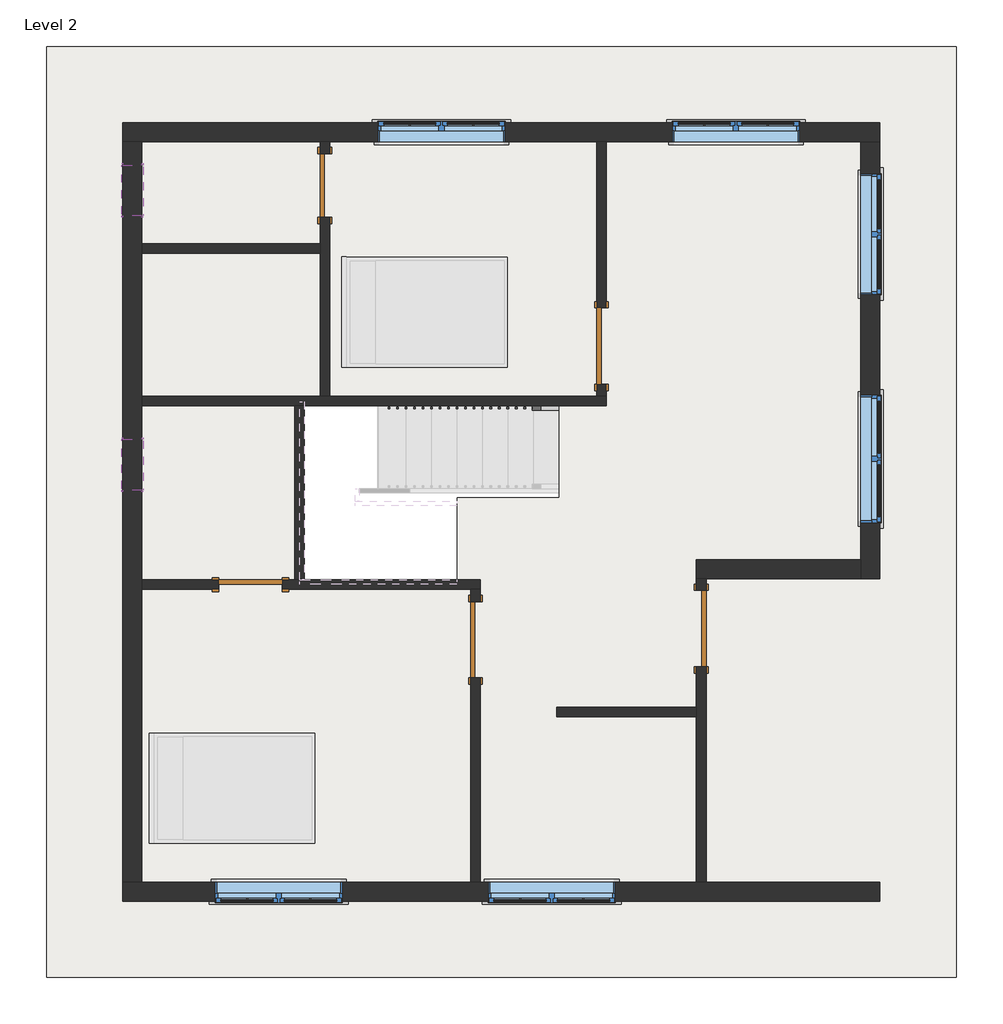
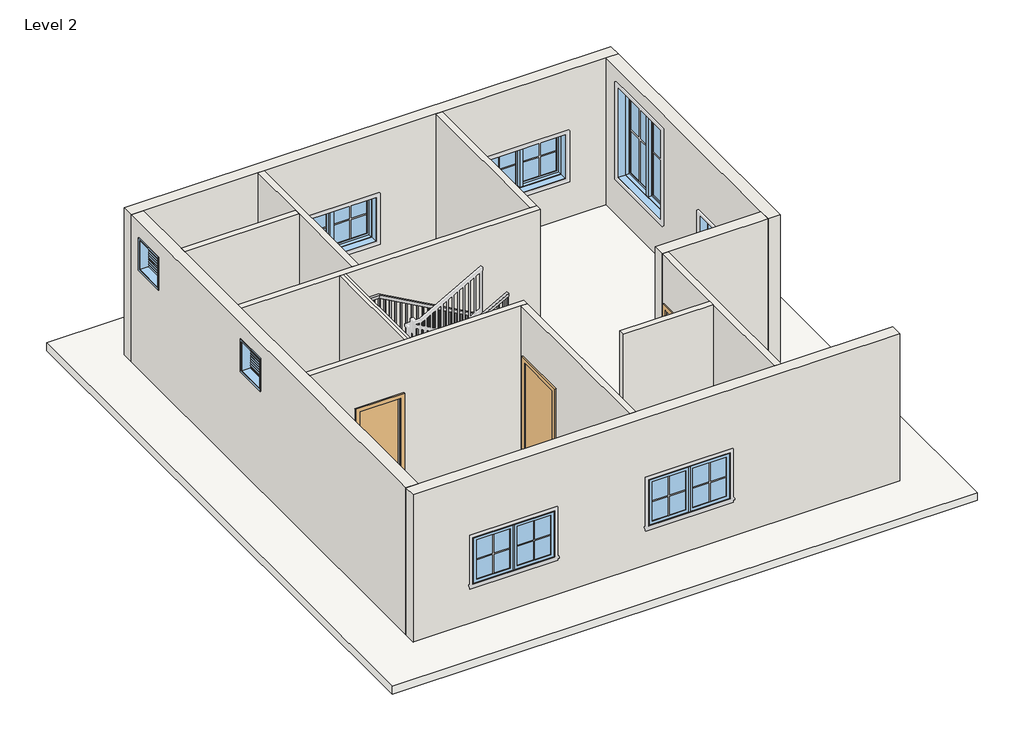
# One storey, part 1 of 2: 14 walls, 8 windows, 5 doors, 1 railing, 1 roof.
"""IFC4 building model written with IfcOpenShell, lengths in millimetres."""

from ifc_helpers import new_model, si_unit, frame, origin, place, context, project, spatial, polyline, outline, extrude, faceted_brep, transform, mapped, element, save
from components import single_flush_3_17d80c48, single_flush_3_5e62189b, door_d8f5dbb5, window_9ac97e1a, window_c1d95f0f, window_f2d8fef0

model = new_model("IFC4")

# Units and contexts
model_context = context("Model", 3, world=origin())
ifc_project = project(units=[si_unit("LENGTHUNIT", "METRE", prefix="MILLI")], contexts=[model_context])

# Site, building, storey
site = spatial("IfcSite", under=ifc_project)
building = spatial("IfcBuilding", under=site)
storey = spatial("IfcBuildingStorey", under=building, Name="Level 2", Elevation=3048.0)

# Doors
placement = place(None, origin())
single_flush_3_shape = single_flush_3_17d80c48(model_context)
element("IfcDoor", 1, ObjectType="Single-Flush : 3'", at=placement, inside=storey, context=model_context, shape_type="MappedRepresentation", body=[
    mapped(single_flush_3_shape, transform((-1566.5130704, -2143.0042021, 3048.0), x_axis=(0.0, 1.0, 0.0), y_axis=(-1.0, 0.0, 0.0), z_axis=(0.0, 0.0, 1.0))),
])
single_flush_3_2_shape = single_flush_3_5e62189b(model_context)
element("IfcDoor", 2, ObjectType="Single-Flush : 3'", at=placement, inside=storey, context=model_context, shape_type="MappedRepresentation", body=[
    mapped(single_flush_3_2_shape, transform((1138.5869296, -2009.6542021, 3048.0), x_axis=(0.0, 1.0, 0.0), y_axis=(-1.0, 0.0, 0.0), z_axis=(0.0, 0.0, 1.0))),
])
element("IfcDoor", 3, ObjectType="Single-Flush : 3'", at=placement, inside=storey, context=model_context, shape_type="MappedRepresentation", body=[
    mapped(single_flush_3_2_shape, transform((-55.2130704, 1374.8957979, 3048.0), x_axis=(0.0, -1.0, 0.0), y_axis=(1.0, 0.0, 0.0), z_axis=(0.0, 0.0, 1.0))),
])
door_shape = door_d8f5dbb5(model_context)
element("IfcDoor", 4, ObjectType="Single-Flush : DOOR 2'6\"", at=placement, inside=storey, context=model_context, shape_type="MappedRepresentation", body=[
    mapped(door_shape, transform((-3369.9130704, 3298.9457979, 3048.0), x_axis=(0.0, 1.0, 0.0), y_axis=(-1.0, 0.0, 0.0), z_axis=(0.0, 0.0, 1.0))),
])
element("IfcDoor", 5, ObjectType="Single-Flush : DOOR 2'6\"", at=placement, inside=storey, context=model_context, shape_type="MappedRepresentation", body=[
    mapped(door_shape, transform((-4258.9130704, -1482.6042021, 3048.0), x_axis=(1.0, 0.0, 0.0), y_axis=(0.0, 1.0, 0.0), z_axis=(0.0, 0.0, 1.0))),
])

# Railing
element("IfcRailing", 6, ObjectType="Handrail - Rectangular", at=placement, inside=storey, context=model_context, shape_type="SolidModel", body=[
    faceted_brep([(-569.5630704, 606.5457979, 4131.7333333), (-569.5630704, 606.5457979, 4073.620221), (-569.5630704, 657.3457979, 4073.620221), (-569.5630704, 657.3457979, 4131.7333333), (-3007.9630704, 606.5457979, 5486.4), (-3021.1266727, 606.5457979, 5435.6), (-3021.1266727, 657.3457979, 5435.6), (-3007.9630704, 657.3457979, 5486.4), (-3566.7630704, 606.5457979, 5486.4), (-3566.7630704, 606.5457979, 5435.6), (-3617.5630704, 657.3457979, 5435.6), (-3617.5630704, 657.3457979, 5486.4), (-3566.7630704, -1374.6542021, 5486.4), (-3566.7630704, -1374.6542021, 5435.6), (-3617.5630704, -1425.4542021, 5435.6), (-3617.5630704, -1425.4542021, 5486.4), (-3312.7630704, -1374.6542021, 5486.4), (-3299.5994682, -1374.6542021, 5435.6), (-3299.5994682, -1425.4542021, 5435.6), (-3312.7630704, -1425.4542021, 5486.4), (-1788.7630704, -1374.6542021, 6333.0666667), (-1788.7630704, -1425.4542021, 6333.0666667), (-1788.7630704, -1425.4542021, 6274.9535543), (-1788.7630704, -1374.6542021, 6274.9535543)], [[[0, 1, 2, 3]], [[1, 0, 4, 5]], [[2, 1, 5, 6]], [[3, 2, 6, 7]], [[0, 3, 7, 4]], [[5, 4, 8, 9]], [[6, 5, 9, 10]], [[7, 6, 10, 11]], [[4, 7, 11, 8]], [[9, 8, 12, 13]], [[10, 9, 13, 14]], [[11, 10, 14, 15]], [[8, 11, 15, 12]], [[13, 12, 16, 17]], [[14, 13, 17, 18]], [[15, 14, 18, 19]], [[12, 15, 19, 16]], [[20, 21, 22, 23]], [[17, 16, 20, 23]], [[18, 17, 23, 22]], [[19, 18, 22, 21]], [[16, 19, 21, 20]]]),
    extrude(outline(polyline([(6237.9118876, -1855.4380704), (6227.3285543, -1874.4880704), (5249.3333333, -1874.4880704), (5249.3333333, -1855.4380704), (6237.9118876, -1855.4380704)])), frame((0.0, -1409.5792021, 0.0), z_axis=(0.0, 1.0, 0.0), x_axis=(0.0, 0.0, 1.0)), (0.0, 0.0, 1.0), 19.05),
    extrude(outline(polyline([(6181.4674432, -1957.0380704), (6170.8841099, -1976.0880704), (5249.3333333, -1976.0880704), (5249.3333333, -1957.0380704), (6181.4674432, -1957.0380704)])), frame((0.0, -1409.5792021, 0.0), z_axis=(0.0, 1.0, 0.0), x_axis=(0.0, 0.0, 1.0)), (0.0, 0.0, 1.0), 19.05),
    extrude(outline(polyline([(6125.0229988, -2058.6380704), (6114.4396654, -2077.6880704), (5249.3333333, -2077.6880704), (5249.3333333, -2058.6380704), (6125.0229988, -2058.6380704)])), frame((0.0, -1409.5792021, 0.0), z_axis=(0.0, 1.0, 0.0), x_axis=(0.0, 0.0, 1.0)), (0.0, 0.0, 1.0), 19.05),
    extrude(outline(polyline([(6068.5785543, -2160.2380704), (6057.995221, -2179.2880704), (5080.0, -2179.2880704), (5080.0, -2160.2380704), (6068.5785543, -2160.2380704)])), frame((0.0, -1409.5792021, 0.0), z_axis=(0.0, 1.0, 0.0), x_axis=(0.0, 0.0, 1.0)), (0.0, 0.0, 1.0), 19.05),
    extrude(outline(polyline([(6012.1341099, -2261.8380704), (6001.5507765, -2280.8880704), (5080.0, -2280.8880704), (5080.0, -2261.8380704), (6012.1341099, -2261.8380704)])), frame((0.0, -1409.5792021, 0.0), z_axis=(0.0, 1.0, 0.0), x_axis=(0.0, 0.0, 1.0)), (0.0, 0.0, 1.0), 19.05),
    extrude(outline(polyline([(5955.6896654, -2363.4380704), (5945.1063321, -2382.4880704), (5080.0, -2382.4880704), (5080.0, -2363.4380704), (5955.6896654, -2363.4380704)])), frame((0.0, -1409.5792021, 0.0), z_axis=(0.0, 1.0, 0.0), x_axis=(0.0, 0.0, 1.0)), (0.0, 0.0, 1.0), 19.05),
    extrude(outline(polyline([(5899.245221, -2465.0380704), (5888.6618876, -2484.0880704), (4910.6666667, -2484.0880704), (4910.6666667, -2465.0380704), (5899.245221, -2465.0380704)])), frame((0.0, -1409.5792021, 0.0), z_axis=(0.0, 1.0, 0.0), x_axis=(0.0, 0.0, 1.0)), (0.0, 0.0, 1.0), 19.05),
    extrude(outline(polyline([(5842.8007765, -2566.6380704), (5832.2174432, -2585.6880704), (4910.6666667, -2585.6880704), (4910.6666667, -2566.6380704), (5842.8007765, -2566.6380704)])), frame((0.0, -1409.5792021, 0.0), z_axis=(0.0, 1.0, 0.0), x_axis=(0.0, 0.0, 1.0)), (0.0, 0.0, 1.0), 19.05),
    extrude(outline(polyline([(5786.3563321, -2668.2380704), (5775.7729988, -2687.2880704), (4910.6666667, -2687.2880704), (4910.6666667, -2668.2380704), (5786.3563321, -2668.2380704)])), frame((0.0, -1409.5792021, 0.0), z_axis=(0.0, 1.0, 0.0), x_axis=(0.0, 0.0, 1.0)), (0.0, 0.0, 1.0), 19.05),
    extrude(outline(polyline([(5729.9118876, -2769.8380704), (5719.3285543, -2788.8880704), (4741.3333333, -2788.8880704), (4741.3333333, -2769.8380704), (5729.9118876, -2769.8380704)])), frame((0.0, -1409.5792021, 0.0), z_axis=(0.0, 1.0, 0.0), x_axis=(0.0, 0.0, 1.0)), (0.0, 0.0, 1.0), 19.05),
    extrude(outline(polyline([(5673.4674432, -2871.4380704), (5662.8841099, -2890.4880704), (4741.3333333, -2890.4880704), (4741.3333333, -2871.4380704), (5673.4674432, -2871.4380704)])), frame((0.0, -1409.5792021, 0.0), z_axis=(0.0, 1.0, 0.0), x_axis=(0.0, 0.0, 1.0)), (0.0, 0.0, 1.0), 19.05),
    extrude(outline(polyline([(5617.0229988, -2973.0380704), (5606.4396654, -2992.0880704), (4741.3333333, -2992.0880704), (4741.3333333, -2973.0380704), (5617.0229988, -2973.0380704)])), frame((0.0, -1409.5792021, 0.0), z_axis=(0.0, 1.0, 0.0), x_axis=(0.0, 0.0, 1.0)), (0.0, 0.0, 1.0), 19.05),
    extrude(outline(polyline([(5560.5785543, -3074.6380704), (5549.995221, -3093.6880704), (4572.0, -3093.6880704), (4572.0, -3074.6380704), (5560.5785543, -3074.6380704)])), frame((0.0, -1409.5792021, 0.0), z_axis=(0.0, 1.0, 0.0), x_axis=(0.0, 0.0, 1.0)), (0.0, 0.0, 1.0), 19.05),
    extrude(outline(polyline([(5504.1341099, -3176.2380704), (5493.5507765, -3195.2880704), (4572.0, -3195.2880704), (4572.0, -3176.2380704), (5504.1341099, -3176.2380704)])), frame((0.0, -1409.5792021, 0.0), z_axis=(0.0, 1.0, 0.0), x_axis=(0.0, 0.0, 1.0)), (0.0, 0.0, 1.0), 19.05),
    extrude(outline(polyline([(5447.6896654, -3277.8380704), (5437.1063321, -3296.8880704), (4572.0, -3296.8880704), (4572.0, -3277.8380704), (5447.6896654, -3277.8380704)])), frame((0.0, -1409.5792021, 0.0), z_axis=(0.0, 1.0, 0.0), x_axis=(0.0, 0.0, 1.0)), (0.0, 0.0, 1.0), 19.05),
    extrude(outline(polyline([(-3398.4880704, -1409.5792021), (-3398.4880704, -1390.5292021), (-3379.4380704, -1390.5292021), (-3379.4380704, -1409.5792021), (-3398.4880704, -1409.5792021)])), frame((0.0, 0.0, 4572.0), z_axis=(0.0, 0.0, 1.0), x_axis=(1.0, 0.0, 0.0)), (0.0, 0.0, 1.0), 863.6),
    extrude(outline(polyline([(-3500.0880704, -1409.5792021), (-3500.0880704, -1390.5292021), (-3481.0380704, -1390.5292021), (-3481.0380704, -1409.5792021), (-3500.0880704, -1409.5792021)])), frame((0.0, 0.0, 4572.0), z_axis=(0.0, 0.0, 1.0), x_axis=(1.0, 0.0, 0.0)), (0.0, 0.0, 1.0), 863.6),
    extrude(outline(polyline([(-3601.6880704, -1288.9292021), (-3582.6380704, -1288.9292021), (-3582.6380704, -1307.9792021), (-3601.6880704, -1307.9792021), (-3601.6880704, -1288.9292021)])), frame((0.0, 0.0, 4572.0), z_axis=(0.0, 0.0, 1.0), x_axis=(1.0, 0.0, 0.0)), (0.0, 0.0, 1.0), 863.6),
    extrude(outline(polyline([(-3601.6880704, -1187.3292021), (-3582.6380704, -1187.3292021), (-3582.6380704, -1206.3792021), (-3601.6880704, -1206.3792021), (-3601.6880704, -1187.3292021)])), frame((0.0, 0.0, 4572.0), z_axis=(0.0, 0.0, 1.0), x_axis=(1.0, 0.0, 0.0)), (0.0, 0.0, 1.0), 863.6),
    extrude(outline(polyline([(-3601.6880704, -1085.7292021), (-3582.6380704, -1085.7292021), (-3582.6380704, -1104.7792021), (-3601.6880704, -1104.7792021), (-3601.6880704, -1085.7292021)])), frame((0.0, 0.0, 4572.0), z_axis=(0.0, 0.0, 1.0), x_axis=(1.0, 0.0, 0.0)), (0.0, 0.0, 1.0), 863.6),
    extrude(outline(polyline([(-3601.6880704, -984.1292021), (-3582.6380704, -984.1292021), (-3582.6380704, -1003.1792021), (-3601.6880704, -1003.1792021), (-3601.6880704, -984.1292021)])), frame((0.0, 0.0, 4572.0), z_axis=(0.0, 0.0, 1.0), x_axis=(1.0, 0.0, 0.0)), (0.0, 0.0, 1.0), 863.6),
    extrude(outline(polyline([(-3601.6880704, -882.5292021), (-3582.6380704, -882.5292021), (-3582.6380704, -901.5792021), (-3601.6880704, -901.5792021), (-3601.6880704, -882.5292021)])), frame((0.0, 0.0, 4572.0), z_axis=(0.0, 0.0, 1.0), x_axis=(1.0, 0.0, 0.0)), (0.0, 0.0, 1.0), 863.6),
    extrude(outline(polyline([(-3601.6880704, -780.9292021), (-3582.6380704, -780.9292021), (-3582.6380704, -799.9792021), (-3601.6880704, -799.9792021), (-3601.6880704, -780.9292021)])), frame((0.0, 0.0, 4572.0), z_axis=(0.0, 0.0, 1.0), x_axis=(1.0, 0.0, 0.0)), (0.0, 0.0, 1.0), 863.6),
    extrude(outline(polyline([(-3601.6880704, -679.3292021), (-3582.6380704, -679.3292021), (-3582.6380704, -698.3792021), (-3601.6880704, -698.3792021), (-3601.6880704, -679.3292021)])), frame((0.0, 0.0, 4572.0), z_axis=(0.0, 0.0, 1.0), x_axis=(1.0, 0.0, 0.0)), (0.0, 0.0, 1.0), 863.6),
    extrude(outline(polyline([(-3601.6880704, -577.7292021), (-3582.6380704, -577.7292021), (-3582.6380704, -596.7792021), (-3601.6880704, -596.7792021), (-3601.6880704, -577.7292021)])), frame((0.0, 0.0, 4572.0), z_axis=(0.0, 0.0, 1.0), x_axis=(1.0, 0.0, 0.0)), (0.0, 0.0, 1.0), 863.6),
    extrude(outline(polyline([(-3601.6880704, -476.1292021), (-3582.6380704, -476.1292021), (-3582.6380704, -495.1792021), (-3601.6880704, -495.1792021), (-3601.6880704, -476.1292021)])), frame((0.0, 0.0, 4572.0), z_axis=(0.0, 0.0, 1.0), x_axis=(1.0, 0.0, 0.0)), (0.0, 0.0, 1.0), 863.6),
    extrude(outline(polyline([(-3601.6880704, -374.5292021), (-3582.6380704, -374.5292021), (-3582.6380704, -393.5792021), (-3601.6880704, -393.5792021), (-3601.6880704, -374.5292021)])), frame((0.0, 0.0, 4572.0), z_axis=(0.0, 0.0, 1.0), x_axis=(1.0, 0.0, 0.0)), (0.0, 0.0, 1.0), 863.6),
    extrude(outline(polyline([(-3601.6880704, -272.9292021), (-3582.6380704, -272.9292021), (-3582.6380704, -291.9792021), (-3601.6880704, -291.9792021), (-3601.6880704, -272.9292021)])), frame((0.0, 0.0, 4572.0), z_axis=(0.0, 0.0, 1.0), x_axis=(1.0, 0.0, 0.0)), (0.0, 0.0, 1.0), 863.6),
    extrude(outline(polyline([(-3601.6880704, -171.3292021), (-3582.6380704, -171.3292021), (-3582.6380704, -190.3792021), (-3601.6880704, -190.3792021), (-3601.6880704, -171.3292021)])), frame((0.0, 0.0, 4572.0), z_axis=(0.0, 0.0, 1.0), x_axis=(1.0, 0.0, 0.0)), (0.0, 0.0, 1.0), 863.6),
    extrude(outline(polyline([(-3601.6880704, -69.7292021), (-3582.6380704, -69.7292021), (-3582.6380704, -88.7792021), (-3601.6880704, -88.7792021), (-3601.6880704, -69.7292021)])), frame((0.0, 0.0, 4572.0), z_axis=(0.0, 0.0, 1.0), x_axis=(1.0, 0.0, 0.0)), (0.0, 0.0, 1.0), 863.6),
    extrude(outline(polyline([(-3601.6880704, 31.8707979), (-3582.6380704, 31.8707979), (-3582.6380704, 12.8207979), (-3601.6880704, 12.8207979), (-3601.6880704, 31.8707979)])), frame((0.0, 0.0, 4572.0), z_axis=(0.0, 0.0, 1.0), x_axis=(1.0, 0.0, 0.0)), (0.0, 0.0, 1.0), 863.6),
    extrude(outline(polyline([(-3601.6880704, 133.4707979), (-3582.6380704, 133.4707979), (-3582.6380704, 114.4207979), (-3601.6880704, 114.4207979), (-3601.6880704, 133.4707979)])), frame((0.0, 0.0, 4572.0), z_axis=(0.0, 0.0, 1.0), x_axis=(1.0, 0.0, 0.0)), (0.0, 0.0, 1.0), 863.6),
    extrude(outline(polyline([(-3601.6880704, 235.0707979), (-3582.6380704, 235.0707979), (-3582.6380704, 216.0207979), (-3601.6880704, 216.0207979), (-3601.6880704, 235.0707979)])), frame((0.0, 0.0, 4572.0), z_axis=(0.0, 0.0, 1.0), x_axis=(1.0, 0.0, 0.0)), (0.0, 0.0, 1.0), 863.6),
    extrude(outline(polyline([(-3601.6880704, 336.6707979), (-3582.6380704, 336.6707979), (-3582.6380704, 317.6207979), (-3601.6880704, 317.6207979), (-3601.6880704, 336.6707979)])), frame((0.0, 0.0, 4572.0), z_axis=(0.0, 0.0, 1.0), x_axis=(1.0, 0.0, 0.0)), (0.0, 0.0, 1.0), 863.6),
    extrude(outline(polyline([(-3601.6880704, 438.2707979), (-3582.6380704, 438.2707979), (-3582.6380704, 419.2207979), (-3601.6880704, 419.2207979), (-3601.6880704, 438.2707979)])), frame((0.0, 0.0, 4572.0), z_axis=(0.0, 0.0, 1.0), x_axis=(1.0, 0.0, 0.0)), (0.0, 0.0, 1.0), 863.6),
    extrude(outline(polyline([(-3601.6880704, 539.8707979), (-3582.6380704, 539.8707979), (-3582.6380704, 520.8207979), (-3601.6880704, 520.8207979), (-3601.6880704, 539.8707979)])), frame((0.0, 0.0, 4572.0), z_axis=(0.0, 0.0, 1.0), x_axis=(1.0, 0.0, 0.0)), (0.0, 0.0, 1.0), 863.6),
    extrude(outline(polyline([(-3506.4380704, 641.4707979), (-3506.4380704, 622.4207979), (-3525.4880704, 622.4207979), (-3525.4880704, 641.4707979), (-3506.4380704, 641.4707979)])), frame((0.0, 0.0, 4572.0), z_axis=(0.0, 0.0, 1.0), x_axis=(1.0, 0.0, 0.0)), (0.0, 0.0, 1.0), 863.6),
    extrude(outline(polyline([(-3404.8380704, 641.4707979), (-3404.8380704, 622.4207979), (-3423.8880704, 622.4207979), (-3423.8880704, 641.4707979), (-3404.8380704, 641.4707979)])), frame((0.0, 0.0, 4572.0), z_axis=(0.0, 0.0, 1.0), x_axis=(1.0, 0.0, 0.0)), (0.0, 0.0, 1.0), 863.6),
    extrude(outline(polyline([(-3303.2380704, 641.4707979), (-3303.2380704, 622.4207979), (-3322.2880704, 622.4207979), (-3322.2880704, 641.4707979), (-3303.2380704, 641.4707979)])), frame((0.0, 0.0, 4572.0), z_axis=(0.0, 0.0, 1.0), x_axis=(1.0, 0.0, 0.0)), (0.0, 0.0, 1.0), 863.6),
    extrude(outline(polyline([(-3201.6380704, 641.4707979), (-3201.6380704, 622.4207979), (-3220.6880704, 622.4207979), (-3220.6880704, 641.4707979), (-3201.6380704, 641.4707979)])), frame((0.0, 0.0, 4572.0), z_axis=(0.0, 0.0, 1.0), x_axis=(1.0, 0.0, 0.0)), (0.0, 0.0, 1.0), 863.6),
    extrude(outline(polyline([(-3100.0380704, 641.4707979), (-3100.0380704, 622.4207979), (-3119.0880704, 622.4207979), (-3119.0880704, 641.4707979), (-3100.0380704, 641.4707979)])), frame((0.0, 0.0, 4572.0), z_axis=(0.0, 0.0, 1.0), x_axis=(1.0, 0.0, 0.0)), (0.0, 0.0, 1.0), 863.6),
    extrude(outline(polyline([(5422.995221, -2998.4380704), (5433.5785543, -3017.4880704), (4572.0, -3017.4880704), (4572.0, -2998.4380704), (5422.995221, -2998.4380704)])), frame((0.0, 622.4207979, 0.0), z_axis=(0.0, 1.0, 0.0), x_axis=(0.0, 0.0, 1.0)), (0.0, 0.0, 1.0), 19.05),
    extrude(outline(polyline([(5366.5507765, -2896.8380704), (5377.1341099, -2915.8880704), (4402.6666667, -2915.8880704), (4402.6666667, -2896.8380704), (5366.5507765, -2896.8380704)])), frame((0.0, 622.4207979, 0.0), z_axis=(0.0, 1.0, 0.0), x_axis=(0.0, 0.0, 1.0)), (0.0, 0.0, 1.0), 19.05),
    extrude(outline(polyline([(5310.1063321, -2795.2380704), (5320.6896654, -2814.2880704), (4402.6666667, -2814.2880704), (4402.6666667, -2795.2380704), (5310.1063321, -2795.2380704)])), frame((0.0, 622.4207979, 0.0), z_axis=(0.0, 1.0, 0.0), x_axis=(0.0, 0.0, 1.0)), (0.0, 0.0, 1.0), 19.05),
    extrude(outline(polyline([(5253.6618876, -2693.6380704), (5264.245221, -2712.6880704), (4402.6666667, -2712.6880704), (4402.6666667, -2693.6380704), (5253.6618876, -2693.6380704)])), frame((0.0, 622.4207979, 0.0), z_axis=(0.0, 1.0, 0.0), x_axis=(0.0, 0.0, 1.0)), (0.0, 0.0, 1.0), 19.05),
    extrude(outline(polyline([(5197.2174432, -2592.0380704), (5207.8007765, -2611.0880704), (4233.3333333, -2611.0880704), (4233.3333333, -2592.0380704), (5197.2174432, -2592.0380704)])), frame((0.0, 622.4207979, 0.0), z_axis=(0.0, 1.0, 0.0), x_axis=(0.0, 0.0, 1.0)), (0.0, 0.0, 1.0), 19.05),
    extrude(outline(polyline([(5140.7729988, -2490.4380704), (5151.3563321, -2509.4880704), (4233.3333333, -2509.4880704), (4233.3333333, -2490.4380704), (5140.7729988, -2490.4380704)])), frame((0.0, 622.4207979, 0.0), z_axis=(0.0, 1.0, 0.0), x_axis=(0.0, 0.0, 1.0)), (0.0, 0.0, 1.0), 19.05),
    extrude(outline(polyline([(5084.3285543, -2388.8380704), (5094.9118876, -2407.8880704), (4233.3333333, -2407.8880704), (4233.3333333, -2388.8380704), (5084.3285543, -2388.8380704)])), frame((0.0, 622.4207979, 0.0), z_axis=(0.0, 1.0, 0.0), x_axis=(0.0, 0.0, 1.0)), (0.0, 0.0, 1.0), 19.05),
    extrude(outline(polyline([(5027.8841099, -2287.2380704), (5038.4674432, -2306.2880704), (4064.0, -2306.2880704), (4064.0, -2287.2380704), (5027.8841099, -2287.2380704)])), frame((0.0, 622.4207979, 0.0), z_axis=(0.0, 1.0, 0.0), x_axis=(0.0, 0.0, 1.0)), (0.0, 0.0, 1.0), 19.05),
    extrude(outline(polyline([(4971.4396654, -2185.6380704), (4982.0229988, -2204.6880704), (4064.0, -2204.6880704), (4064.0, -2185.6380704), (4971.4396654, -2185.6380704)])), frame((0.0, 622.4207979, 0.0), z_axis=(0.0, 1.0, 0.0), x_axis=(0.0, 0.0, 1.0)), (0.0, 0.0, 1.0), 19.05),
    extrude(outline(polyline([(4914.995221, -2084.0380704), (4925.5785543, -2103.0880704), (4064.0, -2103.0880704), (4064.0, -2084.0380704), (4914.995221, -2084.0380704)])), frame((0.0, 622.4207979, 0.0), z_axis=(0.0, 1.0, 0.0), x_axis=(0.0, 0.0, 1.0)), (0.0, 0.0, 1.0), 19.05),
    extrude(outline(polyline([(4858.5507765, -1982.4380704), (4869.1341099, -2001.4880704), (3894.6666667, -2001.4880704), (3894.6666667, -1982.4380704), (4858.5507765, -1982.4380704)])), frame((0.0, 622.4207979, 0.0), z_axis=(0.0, 1.0, 0.0), x_axis=(0.0, 0.0, 1.0)), (0.0, 0.0, 1.0), 19.05),
    extrude(outline(polyline([(4802.1063321, -1880.8380704), (4812.6896654, -1899.8880704), (3894.6666667, -1899.8880704), (3894.6666667, -1880.8380704), (4802.1063321, -1880.8380704)])), frame((0.0, 622.4207979, 0.0), z_axis=(0.0, 1.0, 0.0), x_axis=(0.0, 0.0, 1.0)), (0.0, 0.0, 1.0), 19.05),
    extrude(outline(polyline([(4745.6618876, -1779.2380704), (4756.245221, -1798.2880704), (3894.6666667, -1798.2880704), (3894.6666667, -1779.2380704), (4745.6618876, -1779.2380704)])), frame((0.0, 622.4207979, 0.0), z_axis=(0.0, 1.0, 0.0), x_axis=(0.0, 0.0, 1.0)), (0.0, 0.0, 1.0), 19.05),
    extrude(outline(polyline([(4689.2174432, -1677.6380704), (4699.8007765, -1696.6880704), (3725.3333333, -1696.6880704), (3725.3333333, -1677.6380704), (4689.2174432, -1677.6380704)])), frame((0.0, 622.4207979, 0.0), z_axis=(0.0, 1.0, 0.0), x_axis=(0.0, 0.0, 1.0)), (0.0, 0.0, 1.0), 19.05),
    extrude(outline(polyline([(4632.7729988, -1576.0380704), (4643.3563321, -1595.0880704), (3725.3333333, -1595.0880704), (3725.3333333, -1576.0380704), (4632.7729988, -1576.0380704)])), frame((0.0, 622.4207979, 0.0), z_axis=(0.0, 1.0, 0.0), x_axis=(0.0, 0.0, 1.0)), (0.0, 0.0, 1.0), 19.05),
    extrude(outline(polyline([(4576.3285543, -1474.4380704), (4586.9118876, -1493.4880704), (3725.3333333, -1493.4880704), (3725.3333333, -1474.4380704), (4576.3285543, -1474.4380704)])), frame((0.0, 622.4207979, 0.0), z_axis=(0.0, 1.0, 0.0), x_axis=(0.0, 0.0, 1.0)), (0.0, 0.0, 1.0), 19.05),
    extrude(outline(polyline([(4519.8841099, -1372.8380704), (4530.4674432, -1391.8880704), (3556.0, -1391.8880704), (3556.0, -1372.8380704), (4519.8841099, -1372.8380704)])), frame((0.0, 622.4207979, 0.0), z_axis=(0.0, 1.0, 0.0), x_axis=(0.0, 0.0, 1.0)), (0.0, 0.0, 1.0), 19.05),
    extrude(outline(polyline([(4463.4396654, -1271.2380704), (4474.0229988, -1290.2880704), (3556.0, -1290.2880704), (3556.0, -1271.2380704), (4463.4396654, -1271.2380704)])), frame((0.0, 622.4207979, 0.0), z_axis=(0.0, 1.0, 0.0), x_axis=(0.0, 0.0, 1.0)), (0.0, 0.0, 1.0), 19.05),
    extrude(outline(polyline([(4406.995221, -1169.6380704), (4417.5785543, -1188.6880704), (3556.0, -1188.6880704), (3556.0, -1169.6380704), (4406.995221, -1169.6380704)])), frame((0.0, 622.4207979, 0.0), z_axis=(0.0, 1.0, 0.0), x_axis=(0.0, 0.0, 1.0)), (0.0, 0.0, 1.0), 19.05),
    extrude(outline(polyline([(4350.5507765, -1068.0380704), (4361.1341099, -1087.0880704), (3386.6666667, -1087.0880704), (3386.6666667, -1068.0380704), (4350.5507765, -1068.0380704)])), frame((0.0, 622.4207979, 0.0), z_axis=(0.0, 1.0, 0.0), x_axis=(0.0, 0.0, 1.0)), (0.0, 0.0, 1.0), 19.05),
    extrude(outline(polyline([(4294.1063321, -966.4380704), (4304.6896654, -985.4880704), (3386.6666667, -985.4880704), (3386.6666667, -966.4380704), (4294.1063321, -966.4380704)])), frame((0.0, 622.4207979, 0.0), z_axis=(0.0, 1.0, 0.0), x_axis=(0.0, 0.0, 1.0)), (0.0, 0.0, 1.0), 19.05),
    extrude(outline(polyline([(4237.6618876, -864.8380704), (4248.245221, -883.8880704), (3386.6666667, -883.8880704), (3386.6666667, -864.8380704), (4237.6618876, -864.8380704)])), frame((0.0, 622.4207979, 0.0), z_axis=(0.0, 1.0, 0.0), x_axis=(0.0, 0.0, 1.0)), (0.0, 0.0, 1.0), 19.05),
    extrude(outline(polyline([(4181.2174432, -763.2380704), (4191.8007765, -782.2880704), (3217.3333333, -782.2880704), (3217.3333333, -763.2380704), (4181.2174432, -763.2380704)])), frame((0.0, 622.4207979, 0.0), z_axis=(0.0, 1.0, 0.0), x_axis=(0.0, 0.0, 1.0)), (0.0, 0.0, 1.0), 19.05),
    extrude(outline(polyline([(4124.7729988, -661.6380704), (4135.3563321, -680.6880704), (3217.3333333, -680.6880704), (3217.3333333, -661.6380704), (4124.7729988, -661.6380704)])), frame((0.0, 622.4207979, 0.0), z_axis=(0.0, 1.0, 0.0), x_axis=(0.0, 0.0, 1.0)), (0.0, 0.0, 1.0), 19.05),
    extrude(outline(polyline([(-3601.6880704, -1390.5292021), (-3582.6380704, -1390.5292021), (-3582.6380704, -1409.5792021), (-3601.6880704, -1409.5792021), (-3601.6880704, -1390.5292021)])), frame((0.0, 0.0, 4572.0), z_axis=(0.0, 0.0, 1.0), x_axis=(1.0, 0.0, 0.0)), (0.0, 0.0, 1.0), 863.6),
    extrude(outline(polyline([(-3582.6380704, 641.4707979), (-3582.6380704, 622.4207979), (-3601.6880704, 622.4207979), (-3601.6880704, 641.4707979), (-3582.6380704, 641.4707979)])), frame((0.0, 0.0, 4572.0), z_axis=(0.0, 0.0, 1.0), x_axis=(1.0, 0.0, 0.0)), (0.0, 0.0, 1.0), 863.6),
    extrude(outline(polyline([(6274.9535543, -1788.7630704), (6264.370221, -1807.8130704), (5249.3333333, -1807.8130704), (5249.3333333, -1788.7630704), (6274.9535543, -1788.7630704)])), frame((0.0, -1409.5792021, 0.0), z_axis=(0.0, 1.0, 0.0), x_axis=(0.0, 0.0, 1.0)), (0.0, 0.0, 1.0), 19.05),
    extrude(outline(polyline([(4073.620221, -569.5630704), (4084.2035543, -588.6130704), (3217.3333333, -588.6130704), (3217.3333333, -569.5630704), (4073.620221, -569.5630704)])), frame((0.0, 622.4207979, 0.0), z_axis=(0.0, 1.0, 0.0), x_axis=(0.0, 0.0, 1.0)), (0.0, 0.0, 1.0), 19.05),
])

# Roof
element("IfcRoof", 7, ObjectType="roof 6\"", at=placement, inside=storey, context=model_context, shape_type="SweptSolid", body=[
    extrude(outline(polyline([(4192.9369296, 4962.6457979), (4192.9369296, -6187.9542021), (-6703.6630704, -6187.9542021), (-6703.6630704, 4962.6457979), (4192.9369296, 4962.6457979)]), holes=[polyline([(-3668.3630704, 708.1457979), (-3668.3630704, -1476.2542021), (-1788.7630704, -1476.2542021), (-1788.7630704, -434.8542021), (-569.5630704, -434.8542021), (-569.5630704, 708.1457979), (-3668.3630704, 708.1457979)])]), frame((0.0, 0.0, 3048.0), z_axis=(0.0, 0.0, 1.0), x_axis=(1.0, 0.0, 0.0)), (0.0, 0.0, 1.0), 152.4),
])

# Walls
element("IfcWall", 8, ObjectType="WALL 4.5\"", at=placement, inside=storey, context=model_context, shape_type="Brep", body=[
    faceted_brep([(-3427.0630704, 3819.6457979, 3048.0), (-3427.0630704, 3679.9457979, 3048.0), (-3427.0630704, 3679.9457979, 5080.0), (-3427.0630704, 2917.9457979, 5080.0), (-3427.0630704, 2917.9457979, 3048.0), (-3427.0630704, 2600.4457979, 3048.0), (-3427.0630704, 2486.1457979, 3048.0), (-3427.0630704, 771.6457979, 3048.0), (-3427.0630704, 771.6457979, 6096.0), (-3427.0630704, 2486.1457979, 6096.0), (-3427.0630704, 2600.4457979, 6096.0), (-3427.0630704, 3819.6457979, 6096.0), (-3312.7630704, 3679.9457979, 5080.0), (-3312.7630704, 3679.9457979, 3048.0), (-3312.7630704, 3819.6457979, 3048.0), (-3312.7630704, 3819.6457979, 6096.0), (-3312.7630704, 771.6457979, 6096.0), (-3312.7630704, 771.6457979, 3048.0), (-3312.7630704, 2917.9457979, 3048.0), (-3312.7630704, 2917.9457979, 5080.0)], [[[0, 1, 2, 3, 4, 5, 6, 7, 8, 9, 10, 11]], [[12, 13, 14, 15, 16, 17, 18, 19]], [[18, 17, 7, 6, 5, 4]], [[14, 13, 1, 0]], [[0, 11, 15, 14]], [[8, 7, 17, 16]], [[2, 1, 13, 12]], [[3, 2, 12, 19]], [[4, 3, 19, 18]], [[11, 10, 9, 8, 16, 15]]]),
])
element("IfcWall", 9, ObjectType="WALL 4.5\"", at=placement, inside=storey, context=model_context, shape_type="Brep", body=[
    faceted_brep([(-5560.6630704, 657.3457979, 3048.0), (-3731.8630704, 657.3457979, 3048.0), (-3617.5630704, 657.3457979, 3048.0), (1.9369296, 657.3457979, 3048.0), (1.9369296, 657.3457979, 6096.0), (-3617.5630704, 657.3457979, 6096.0), (-3731.8630704, 657.3457979, 6096.0), (-5560.6630704, 657.3457979, 6096.0), (-5560.6630704, 771.6457979, 3048.0), (-5560.6630704, 771.6457979, 6096.0), (-3427.0630704, 771.6457979, 6096.0), (-3312.7630704, 771.6457979, 6096.0), (-112.3630704, 771.6457979, 6096.0), (1.9369296, 771.6457979, 6096.0), (1.9369296, 771.6457979, 3048.0), (-112.3630704, 771.6457979, 3048.0), (-3312.7630704, 771.6457979, 3048.0), (-3427.0630704, 771.6457979, 3048.0)], [[[0, 1, 2, 3, 4, 5, 6, 7]], [[8, 9, 10, 11, 12, 13, 14, 15, 16, 17]], [[3, 2, 1, 0, 8, 17, 16, 15, 14]], [[7, 6, 5, 4, 13, 12, 11, 10, 9]], [[0, 7, 9, 8]], [[4, 3, 14, 13]]]),
])
element("IfcWall", 10, ObjectType="WALL 4.5\"", at=placement, inside=storey, context=model_context, shape_type="SweptSolid", body=[
    extrude(outline(polyline([(917.6957979, 5080.0), (917.6957979, 3048.0), (771.6457979, 3048.0), (771.6457979, 6096.0), (3819.6457979, 6096.0), (3819.6457979, 3048.0), (1832.0957979, 3048.0), (1832.0957979, 5080.0), (917.6957979, 5080.0)])), frame((-112.3630704, 0.0, 0.0), z_axis=(1.0, 0.0, 0.0), x_axis=(0.0, 1.0, 0.0)), (0.0, 0.0, 1.0), 114.3),
])
element("IfcWall", 11, ObjectType="WALL 4.5\"", at=placement, inside=storey, context=model_context, shape_type="SweptSolid", body=[
    extrude(outline(polyline([(-3427.0630704, 2486.1457979), (-5560.6630704, 2486.1457979), (-5560.6630704, 2600.4457979), (-3427.0630704, 2600.4457979), (-3427.0630704, 2486.1457979)])), frame((0.0, 0.0, 3048.0), z_axis=(0.0, 0.0, 1.0), x_axis=(1.0, 0.0, 0.0)), (0.0, 0.0, 1.0), 3048.0),
])
element("IfcWall", 12, ObjectType="WALL 4.5\"", at=placement, inside=storey, context=model_context, shape_type="Brep", body=[
    faceted_brep([(-3877.9130704, -1539.7542021, 5080.0), (-3877.9130704, -1539.7542021, 3048.0), (-1623.6630704, -1539.7542021, 3048.0), (-1509.3630704, -1539.7542021, 3048.0), (-1509.3630704, -1539.7542021, 6096.0), (-1623.6630704, -1539.7542021, 6096.0), (-5560.6630704, -1539.7542021, 6096.0), (-5560.6630704, -1539.7542021, 3048.0), (-4639.9130704, -1539.7542021, 3048.0), (-4639.9130704, -1539.7542021, 5080.0), (-1509.3630704, -1425.4542021, 3048.0), (-3617.5630704, -1425.4542021, 3048.0), (-3731.8630704, -1425.4542021, 3048.0), (-3877.9130704, -1425.4542021, 3048.0), (-3877.9130704, -1425.4542021, 5080.0), (-4639.9130704, -1425.4542021, 5080.0), (-4639.9130704, -1425.4542021, 3048.0), (-5560.6630704, -1425.4542021, 3048.0), (-5560.6630704, -1425.4542021, 6096.0), (-3731.8630704, -1425.4542021, 6096.0), (-3617.5630704, -1425.4542021, 6096.0), (-1509.3630704, -1425.4542021, 6096.0)], [[[0, 1, 2, 3, 4, 5, 6, 7, 8, 9]], [[10, 11, 12, 13, 14, 15, 16, 17, 18, 19, 20, 21]], [[8, 7, 17, 16]], [[3, 2, 1, 13, 12, 11, 10]], [[6, 5, 4, 21, 20, 19, 18]], [[7, 6, 18, 17]], [[4, 3, 10, 21]], [[14, 13, 1, 0]], [[15, 14, 0, 9]], [[16, 15, 9, 8]]]),
])
element("IfcWall", 13, ObjectType="WALL 4.5\"", at=placement, inside=storey, context=model_context, shape_type="SweptSolid", body=[
    extrude(outline(polyline([(-1539.7542021, 3048.0), (-1685.8042021, 3048.0), (-1685.8042021, 5080.0), (-2600.2042021, 5080.0), (-2600.2042021, 3048.0), (-5044.9542021, 3048.0), (-5044.9542021, 6096.0), (-1539.7542021, 6096.0), (-1539.7542021, 3048.0)])), frame((-1623.6630704, 0.0, 0.0), z_axis=(1.0, 0.0, 0.0), x_axis=(0.0, 1.0, 0.0)), (0.0, 0.0, 1.0), 114.3),
])
element("IfcWall", 14, ObjectType="WALL 4.5\"", at=placement, inside=storey, context=model_context, shape_type="Brep", body=[
    faceted_brep([(1195.7369296, -1552.4542021, 5080.0), (1195.7369296, -1552.4542021, 3048.0), (1195.7369296, -1412.7542021, 3048.0), (1195.7369296, -1412.7542021, 6096.0), (1195.7369296, -5044.9542021, 6096.0), (1195.7369296, -5044.9542021, 3048.0), (1195.7369296, -2466.8542021, 3048.0), (1195.7369296, -2466.8542021, 5080.0), (1081.4369296, -1412.7542021, 3048.0), (1081.4369296, -1552.4542021, 3048.0), (1081.4369296, -1552.4542021, 5080.0), (1081.4369296, -2466.8542021, 5080.0), (1081.4369296, -2466.8542021, 3048.0), (1081.4369296, -2948.9967683, 3048.0), (1081.4369296, -3063.2967683, 3048.0), (1081.4369296, -5044.9542021, 3048.0), (1081.4369296, -5044.9542021, 6096.0), (1081.4369296, -3063.2967683, 6096.0), (1081.4369296, -2948.9967683, 6096.0), (1081.4369296, -1412.7542021, 6096.0)], [[[0, 1, 2, 3, 4, 5, 6, 7]], [[8, 9, 10, 11, 12, 13, 14, 15, 16, 17, 18, 19]], [[6, 5, 15, 14, 13, 12]], [[2, 1, 9, 8]], [[3, 2, 8, 19]], [[5, 4, 16, 15]], [[10, 9, 1, 0]], [[11, 10, 0, 7]], [[12, 11, 7, 6]], [[4, 3, 19, 18, 17, 16]]]),
])
element("IfcWall", 15, ObjectType="WALL 4.5\"", at=placement, inside=storey, context=model_context, shape_type="SweptSolid", body=[
    extrude(outline(polyline([(-594.9630704, -2948.9967683), (1081.4369296, -2948.9967683), (1081.4369296, -3063.2967683), (-594.9630704, -3063.2967683), (-594.9630704, -2948.9967683)])), frame((0.0, 0.0, 3048.0), z_axis=(0.0, 0.0, 1.0), x_axis=(1.0, 0.0, 0.0)), (0.0, 0.0, 1.0), 3048.0),
])
element("IfcWall", 16, ObjectType="WALL 4.5\"", at=placement, inside=storey, context=model_context, shape_type="SweptSolid", body=[
    extrude(outline(polyline([(6096.0, -3731.8630704), (3048.0, -3731.8630704), (3048.0, -3617.5630704), (6096.0, -3617.5630704), (6096.0, -3668.3630704), (6096.0, -3731.8630704)])), frame((0.0, -1425.4542021, 0.0), z_axis=(0.0, 1.0, 0.0), x_axis=(0.0, 0.0, 1.0)), (0.0, 0.0, 1.0), 2082.8),
])
element("IfcWall", 17, ObjectType="WALL 9\"", at=placement, inside=storey, context=model_context, shape_type="Brep", body=[
    faceted_brep([(-5789.2630704, 3819.6457979, 3048.0), (-5560.6630704, 3819.6457979, 3048.0), (-3427.0630704, 3819.6457979, 3048.0), (-3312.7630704, 3819.6457979, 3048.0), (-112.3630704, 3819.6457979, 3048.0), (1.9369296, 3819.6457979, 3048.0), (3049.9369296, 3819.6457979, 3048.0), (3278.5369296, 3819.6457979, 3048.0), (3278.5369296, 3819.6457979, 6096.0), (3049.9369296, 3819.6457979, 6096.0), (1.9369296, 3819.6457979, 6096.0), (-112.3630704, 3819.6457979, 6096.0), (-3312.7630704, 3819.6457979, 6096.0), (-3427.0630704, 3819.6457979, 6096.0), (-5560.6630704, 3819.6457979, 6096.0), (-5789.2630704, 3819.6457979, 6096.0), (2316.5119296, 3819.6457979, 4876.8), (2316.5119296, 3819.6457979, 3962.4), (792.5119296, 3819.6457979, 3962.4), (792.5119296, 3819.6457979, 4876.8), (-1210.9130704, 3819.6457979, 4876.8), (-1210.9130704, 3819.6457979, 3962.4), (-2734.9130704, 3819.6457979, 3962.4), (-2734.9130704, 3819.6457979, 4876.8), (-5789.2630704, 4048.2457979, 3048.0), (-5789.2630704, 4048.2457979, 6096.0), (3278.5369296, 4048.2457979, 6096.0), (3278.5369296, 4048.2457979, 3048.0), (2316.5119296, 4048.2457979, 4876.8), (792.5119296, 4048.2457979, 4876.8), (792.5119296, 4048.2457979, 3962.4), (2316.5119296, 4048.2457979, 3962.4), (-1210.9130704, 4048.2457979, 4876.8), (-2734.9130704, 4048.2457979, 4876.8), (-2734.9130704, 4048.2457979, 3962.4), (-1210.9130704, 4048.2457979, 3962.4)], [[[0, 1, 2, 3, 4, 5, 6, 7, 8, 9, 10, 11, 12, 13, 14, 15], [16, 17, 18, 19], [20, 21, 22, 23]], [[24, 25, 26, 27], [28, 29, 30, 31], [32, 33, 34, 35]], [[7, 6, 5, 4, 3, 2, 1, 0, 24, 27]], [[8, 7, 27, 26]], [[0, 15, 25, 24]], [[17, 16, 28, 31]], [[18, 17, 31, 30]], [[19, 18, 30, 29]], [[16, 19, 29, 28]], [[21, 20, 32, 35]], [[22, 21, 35, 34]], [[23, 22, 34, 33]], [[20, 23, 33, 32]], [[15, 14, 13, 12, 11, 10, 9, 8, 26, 25]]]),
])
element("IfcWall", 18, ObjectType="WALL 9\"", at=placement, inside=storey, context=model_context, shape_type="Brep", body=[
    faceted_brep([(3049.9369296, 3819.6457979, 3048.0), (3049.9369296, -1184.1542021, 3048.0), (3049.9369296, -1412.7542021, 3048.0), (3049.9369296, -1412.7542021, 6096.0), (3049.9369296, -1184.1542021, 6096.0), (3049.9369296, 3819.6457979, 6096.0), (3049.9369296, -739.6542021, 4876.8), (3049.9369296, -739.6542021, 3962.4), (3049.9369296, 784.3457979, 3962.4), (3049.9369296, 784.3457979, 4876.8), (3049.9369296, 1990.8457979, 5791.2), (3049.9369296, 1990.8457979, 3962.4), (3049.9369296, 3438.6457979, 3962.4), (3049.9369296, 3438.6457979, 5791.2), (3278.5369296, 3819.6457979, 3048.0), (3278.5369296, 3819.6457979, 6096.0), (3278.5369296, -1412.7542021, 6096.0), (3278.5369296, -1412.7542021, 3048.0), (3278.5369296, -739.6542021, 4876.8), (3278.5369296, 784.3457979, 4876.8), (3278.5369296, 784.3457979, 3962.4), (3278.5369296, -739.6542021, 3962.4), (3278.5369296, 1990.8457979, 5791.2), (3278.5369296, 3438.6457979, 5791.2), (3278.5369296, 3438.6457979, 3962.4), (3278.5369296, 1990.8457979, 3962.4)], [[[0, 1, 2, 3, 4, 5], [6, 7, 8, 9], [10, 11, 12, 13]], [[14, 15, 16, 17], [18, 19, 20, 21], [22, 23, 24, 25]], [[2, 1, 0, 14, 17]], [[0, 5, 15, 14]], [[3, 2, 17, 16]], [[7, 6, 18, 21]], [[8, 7, 21, 20]], [[9, 8, 20, 19]], [[6, 9, 19, 18]], [[11, 10, 22, 25]], [[12, 11, 25, 24]], [[13, 12, 24, 23]], [[10, 13, 23, 22]], [[5, 4, 3, 16, 15]]]),
])
element("IfcWall", 19, ObjectType="WALL 9\"", at=placement, inside=storey, context=model_context, shape_type="Brep", body=[
    faceted_brep([(3049.9369296, -1184.1542021, 3048.0), (1081.4369296, -1184.1542021, 3048.0), (1081.4369296, -1184.1542021, 6096.0), (3049.9369296, -1184.1542021, 6096.0), (3049.9369296, -1412.7542021, 3048.0), (3049.9369296, -1412.7542021, 6096.0), (1195.7369296, -1412.7542021, 6096.0), (1081.4369296, -1412.7542021, 6096.0), (1081.4369296, -1412.7542021, 3048.0), (1195.7369296, -1412.7542021, 3048.0)], [[[0, 1, 2, 3]], [[4, 5, 6, 7, 8, 9]], [[1, 0, 4, 9, 8]], [[0, 3, 5, 4]], [[2, 1, 8, 7]], [[3, 2, 7, 6, 5]]]),
])
element("IfcWall", 20, ObjectType="WALL 9\"", at=placement, inside=storey, context=model_context, shape_type="Brep", body=[
    faceted_brep([(3278.5369296, -5044.9542021, 3048.0), (1195.7369296, -5044.9542021, 3048.0), (1081.4369296, -5044.9542021, 3048.0), (-1509.3630704, -5044.9542021, 3048.0), (-1623.6630704, -5044.9542021, 3048.0), (-5560.6630704, -5044.9542021, 3048.0), (-5789.2630704, -5044.9542021, 3048.0), (-5789.2630704, -5044.9542021, 6096.0), (-5560.6630704, -5044.9542021, 6096.0), (-1623.6630704, -5044.9542021, 6096.0), (-1509.3630704, -5044.9542021, 6096.0), (1081.4369296, -5044.9542021, 6096.0), (1195.7369296, -5044.9542021, 6096.0), (3278.5369296, -5044.9542021, 6096.0), (-4684.3630704, -5044.9542021, 4876.8), (-4684.3630704, -5044.9542021, 3962.4), (-3160.3630704, -5044.9542021, 3962.4), (-3160.3630704, -5044.9542021, 4876.8), (-1414.1130704, -5044.9542021, 4876.8), (-1414.1130704, -5044.9542021, 3962.4), (109.8869296, -5044.9542021, 3962.4), (109.8869296, -5044.9542021, 4876.8), (3278.5369296, -5273.5542021, 3048.0), (3278.5369296, -5273.5542021, 6096.0), (-5789.2630704, -5273.5542021, 6096.0), (-5789.2630704, -5273.5542021, 3048.0), (-4684.3630704, -5273.5542021, 4876.8), (-3160.3630704, -5273.5542021, 4876.8), (-3160.3630704, -5273.5542021, 3962.4), (-4684.3630704, -5273.5542021, 3962.4), (-1414.1130704, -5273.5542021, 4876.8), (109.8869296, -5273.5542021, 4876.8), (109.8869296, -5273.5542021, 3962.4), (-1414.1130704, -5273.5542021, 3962.4)], [[[0, 1, 2, 3, 4, 5, 6, 7, 8, 9, 10, 11, 12, 13], [14, 15, 16, 17], [18, 19, 20, 21]], [[22, 23, 24, 25], [26, 27, 28, 29], [30, 31, 32, 33]], [[6, 5, 4, 3, 2, 1, 0, 22, 25]], [[0, 13, 23, 22]], [[7, 6, 25, 24]], [[15, 14, 26, 29]], [[16, 15, 29, 28]], [[17, 16, 28, 27]], [[14, 17, 27, 26]], [[19, 18, 30, 33]], [[20, 19, 33, 32]], [[21, 20, 32, 31]], [[18, 21, 31, 30]], [[13, 12, 11, 10, 9, 8, 7, 24, 23]]]),
])
element("IfcWall", 21, ObjectType="WALL 9\"", at=placement, inside=storey, context=model_context, shape_type="Brep", body=[
    faceted_brep([(-5560.6630704, -5044.9542021, 3048.0), (-5560.6630704, -1539.7542021, 3048.0), (-5560.6630704, -1425.4542021, 3048.0), (-5560.6630704, 657.3457979, 3048.0), (-5560.6630704, 771.6457979, 3048.0), (-5560.6630704, 2486.1457979, 3048.0), (-5560.6630704, 2600.4457979, 3048.0), (-5560.6630704, 3819.6457979, 3048.0), (-5560.6630704, 3819.6457979, 6096.0), (-5560.6630704, 2600.4457979, 6096.0), (-5560.6630704, 2486.1457979, 6096.0), (-5560.6630704, 771.6457979, 6096.0), (-5560.6630704, 657.3457979, 6096.0), (-5560.6630704, -1425.4542021, 6096.0), (-5560.6630704, -1539.7542021, 6096.0), (-5560.6630704, -5044.9542021, 6096.0), (-5560.6630704, 257.2957979, 5791.2), (-5560.6630704, 257.2957979, 5181.6), (-5560.6630704, -352.3042021, 5181.6), (-5560.6630704, -352.3042021, 5791.2), (-5560.6630704, 3543.4207979, 5791.2), (-5560.6630704, 3543.4207979, 5181.6), (-5560.6630704, 2933.8207979, 5181.6), (-5560.6630704, 2933.8207979, 5791.2), (-5789.2630704, -5044.9542021, 3048.0), (-5789.2630704, -5044.9542021, 6096.0), (-5789.2630704, 3819.6457979, 6096.0), (-5789.2630704, 3819.6457979, 3048.0), (-5789.2630704, 257.2957979, 5791.2), (-5789.2630704, -352.3042021, 5791.2), (-5789.2630704, -352.3042021, 5181.6), (-5789.2630704, 257.2957979, 5181.6), (-5789.2630704, 3543.4207979, 5791.2), (-5789.2630704, 2933.8207979, 5791.2), (-5789.2630704, 2933.8207979, 5181.6), (-5789.2630704, 3543.4207979, 5181.6)], [[[0, 1, 2, 3, 4, 5, 6, 7, 8, 9, 10, 11, 12, 13, 14, 15], [16, 17, 18, 19], [20, 21, 22, 23]], [[24, 25, 26, 27], [28, 29, 30, 31], [32, 33, 34, 35]], [[7, 6, 5, 4, 3, 2, 1, 0, 24, 27]], [[0, 15, 25, 24]], [[8, 7, 27, 26]], [[17, 16, 28, 31]], [[18, 17, 31, 30]], [[19, 18, 30, 29]], [[16, 19, 29, 28]], [[21, 20, 32, 35]], [[22, 21, 35, 34]], [[23, 22, 34, 33]], [[20, 23, 33, 32]], [[15, 14, 13, 12, 11, 10, 9, 8, 26, 25]]]),
])

# Windows
window_shape = window_9ac97e1a(model_context)
element("IfcWindow", 22, ObjectType="Window-Casement-Double : 57\" x 72\"", at=placement, inside=storey, context=model_context, shape_type="MappedRepresentation", body=[
    mapped(window_shape, transform((3164.2369296, 2714.7457979, 3048.0), x_axis=(0.0, -1.0, 0.0), y_axis=(1.0, 0.0, 0.0), z_axis=(0.0, 0.0, 1.0))),
])
window_2_shape = window_c1d95f0f(model_context)
element("IfcWindow", 23, ObjectType="Window-Casement-Double : WINDOW 6\"", at=placement, inside=storey, context=model_context, shape_type="MappedRepresentation", body=[
    mapped(window_2_shape, transform((-3922.3630704, -5159.2542021, 3048.0), x_axis=(-1.0, 0.0, 0.0), y_axis=(0.0, -1.0, 0.0), z_axis=(0.0, 0.0, 1.0))),
])
element("IfcWindow", 24, ObjectType="Window-Casement-Double : WINDOW 6\"", at=placement, inside=storey, context=model_context, shape_type="MappedRepresentation", body=[
    mapped(window_2_shape, transform((-652.1130704, -5159.2542021, 3048.0), x_axis=(-1.0, 0.0, 0.0), y_axis=(0.0, -1.0, 0.0), z_axis=(0.0, 0.0, 1.0))),
])
element("IfcWindow", 25, ObjectType="Window-Casement-Double : WINDOW 6\"", at=placement, inside=storey, context=model_context, shape_type="MappedRepresentation", body=[
    mapped(window_2_shape, transform((3164.2369296, 22.3457979, 3048.0), x_axis=(0.0, -1.0, 0.0), y_axis=(1.0, 0.0, 0.0), z_axis=(0.0, 0.0, 1.0))),
])
element("IfcWindow", 26, ObjectType="Window-Casement-Double : WINDOW 6\"", at=placement, inside=storey, context=model_context, shape_type="MappedRepresentation", body=[
    mapped(window_2_shape, transform((1554.5119296, 3933.9457979, 3048.0), x_axis=(1.0, 0.0, 0.0), y_axis=(0.0, 1.0, 0.0), z_axis=(0.0, 0.0, 1.0))),
])
element("IfcWindow", 27, ObjectType="Window-Casement-Double : WINDOW 6\"", at=placement, inside=storey, context=model_context, shape_type="MappedRepresentation", body=[
    mapped(window_2_shape, transform((-1972.9130704, 3933.9457979, 3048.0), x_axis=(1.0, 0.0, 0.0), y_axis=(0.0, 1.0, 0.0), z_axis=(0.0, 0.0, 1.0))),
])
window_3_shape = window_f2d8fef0(model_context)
element("IfcWindow", 28, ObjectType="Window-Louvers : 24\" x 24\"", at=placement, inside=storey, context=model_context, shape_type="MappedRepresentation", body=[
    mapped(window_3_shape, transform((-5668.6130704, -47.5042021, 4267.2), x_axis=(0.0, -1.0, 0.0), y_axis=(1.0, 0.0, 0.0), z_axis=(0.0, 0.0, 1.0))),
])
element("IfcWindow", 29, ObjectType="Window-Louvers : 24\" x 24\"", at=placement, inside=storey, context=model_context, shape_type="MappedRepresentation", body=[
    mapped(window_3_shape, transform((-5668.6130704, 3238.6207979, 4267.2), x_axis=(0.0, -1.0, 0.0), y_axis=(1.0, 0.0, 0.0), z_axis=(0.0, 0.0, 1.0))),
])

save(model, "model.ifc")

# Revit data of these elements
# Type "Single-Flush : 3'"
#   Type Mark = "8"
#   Construction Type Id = "MDOOR"
#   Assembly Code = "C1020"
#   Analytic Construction = "Metal"
#   Thickness = 0' - 2"
#   Heat Transfer Coefficient (U) = 0.651978 BTU/(h·ft²·°F)
#   Height = 6' - 8"
#   Trim Projection Ext = 0' - 1"
#   Trim Projection Int = 0' - 1"
#   Trim Width = 0' - 3"
#   Width = 3' - 0"
#   Define Thermal Properties by = 1
#   Door Material = Door - Panel
#   Frame Material = Door - Frame
#   Visual Light Transmittance = 0
#   Solar Heat Gain Coefficient = 0
#   Function = (empty or 0)
#   Wall Closure = (empty or 0)
# Type "Single-Flush : DOOR 2'6\""
#   Type Mark = "9"
#   Construction Type Id = "MDOOR"
#   Assembly Code = "C1020"
#   Analytic Construction = "Metal"
#   Thickness = 0' - 2"
#   Heat Transfer Coefficient (U) = 0.651978 BTU/(h·ft²·°F)
#   Height = 6' - 8"
#   Trim Projection Ext = 0' - 1"
#   Trim Projection Int = 0' - 1"
#   Trim Width = 0' - 3"
#   Width = 2' - 6"
#   Define Thermal Properties by = 1
#   Door Material = Door - Panel
#   Frame Material = Door - Frame
#   Visual Light Transmittance = 0
#   Solar Heat Gain Coefficient = 0
#   Function = (empty or 0)
#   Wall Closure = (empty or 0)
# Type "Handrail - Rectangular"
#   Assembly Code = "C2010400"
#   built-in parameter 1008612 = 0.0416667 (stored number, unit not read)
#   built-in parameter 1008611 = 0.0416667 (stored number, unit not read)
#   built-in parameter 1008609 = 0.333333 (stored number, unit not read)
#   built-in parameter 1008604 = 0.166667 (stored number, unit not read)
#   built-in parameter 1008603 = 0.166667 (stored number, unit not read)
#   Railing Height = 3' - 0"
#   built-in parameter 1008630 = 2
#   built-in parameter 1008610 = 2
#   built-in parameter 1008618 = Baluster - Square : 3/4"
# Type "roof 6\""
#   Assembly Code = "B1020"
#   Layers, outside or top first: 0' - 6" no material (function 1)
# Type "WALL 4.5\""
#   Assembly Code = "B2010"
#   Layers, outside or top first: 0' - 4 1/2" no material (function 1)
# Type "WALL 9\""
#   Assembly Code = "B2010"
#   Layers, outside or top first: 0' - 9" no material (function 1)
# Type "Window-Casement-Double : 57\" x 72\""
#   Type Mark = "17"
#   Fire Rating = "0.5h"
#   Assembly Code = "B2020100"
#   Analytic Construction = "Double glazing - domestic"
#   Frame Extension [instance default] = 0' - 0 1/4"
#   Window Inset [instance default] = 0' - 0"
#   Wall Thickness [instance default] = 0' - 6"
#   Interior Wall Closure [instance default] = 0' - 2 1/4"
#   Half Width = 2' - 4 1/2"
#   Visual Light Transmittance = 0.81
#   Thermal Resistance (R) = 1.8146 (h·ft²·°F)/BTU
#   Solar Heat Gain Coefficient = 0.76
#   Rough Width = 4' - 9 1/2"
#   Rough Height = 6' - 0 1/2"
#   Height = 6' - 0"
#   Heat Transfer Coefficient (U) = 0.5511 BTU/(h·ft²·°F)
#   Exterior Wall Closure [instance default] = 0' - 1 1/4"
#   Extension Jamb [instance default] = 0' - 2 1/4"
#   Default Sill Height = 3' - 0"
#   Width = 4' - 9"
#   Define Thermal Properties by = 0
#   Muntin Visibility = yes
#   Interior Trim Visibility [instance default] = yes
#   Exterior Trim Visibility [instance default] = yes
#   Extension Jamb Visibility [instance default] = yes
#   Interior Trim Material = Wood - Stained
#   Muntin Pattern = Muntin Pattern_2x2 : Muntin Pattern_2x2
#   Interior Trim = Trim-Window-Interior-Flat : Picture Frame
#   Interior Frame Material = Wood - Stained
#   Glass Panel Material = Glass
#   Exterior Trim Material = Clad - White
#   Exterior Trim = Trim-Window-Exterior-Flat : with Sill
#   Exterior Frame Material = Clad - White
#   Wall Closure = (empty or 0)
# Type "Window-Casement-Double : WINDOW 6\""
#   Type Mark = "18"
#   Fire Rating = "0.5h"
#   Assembly Code = "B2020100"
#   Analytic Construction = "Double glazing - domestic"
#   Frame Extension [instance default] = 0' - 0 1/4"
#   Window Inset [instance default] = 0' - 0"
#   Wall Thickness [instance default] = 0' - 6"
#   Interior Wall Closure [instance default] = 0' - 2 1/4"
#   Half Width = 2' - 6"
#   Visual Light Transmittance = 0.81
#   Thermal Resistance (R) = 1.8146 (h·ft²·°F)/BTU
#   Solar Heat Gain Coefficient = 0.76
#   Rough Width = 5' - 0 1/2"
#   Rough Height = 3' - 0 1/2"
#   Height = 3' - 0"
#   Heat Transfer Coefficient (U) = 0.5511 BTU/(h·ft²·°F)
#   Exterior Wall Closure [instance default] = 0' - 1 1/4"
#   Extension Jamb [instance default] = 0' - 2 1/4"
#   Default Sill Height = 3' - 0"
#   Width = 5' - 0"
#   Muntin Visibility = yes
#   Interior Trim Visibility [instance default] = yes
#   Exterior Trim Visibility [instance default] = yes
#   Extension Jamb Visibility [instance default] = yes
#   Interior Trim Material = Wood - Stained
#   Muntin Pattern = Muntin Pattern_2x2 : Muntin Pattern_2x2
#   Interior Trim = Trim-Window-Interior-Flat : Picture Frame
#   Interior Frame Material = Wood - Stained
#   Glass Panel Material = Glass
#   Exterior Trim Material = Clad - White
#   Exterior Trim = Trim-Window-Exterior-Flat : with Sill
#   Exterior Frame Material = Clad - White
#   Wall Closure = (empty or 0)
# Type "Window-Louvers : 24\" x 24\""
#   Type Mark = "19"
#   Construction Type Id = "GSP4R"
#   Assembly Code = "B20"
#   Analytic Construction = "1/8 in Pilkington single glazing"
#   Visual Light Transmittance = 0.9
#   Thermal Resistance (R) = 1.53941 (h·ft²·°F)/BTU
#   Solar Heat Gain Coefficient = 0.78
#   Max Height = 1' - 11.74264"
#   Height = 2' - 0"
#   Heat Transfer Coefficient (U) = 0.6496 BTU/(h·ft²·°F)
#   Blade Width [instance default] = 1' - 10 1/2"
#   Blade Vertical Thickness = 0' - 0.35355"
#   Blade Thickness = 0' - 0 1/4"
#   Blade Spacing = 0' - 1 1/2"
#   Blade Height = 0' - 1.85355"
#   Blade Depth = 0' - 3"
#   Blade Angle = 45.00°
#   Default Sill Height = 3' - 0"
#   Trim Projection_Exterior = 0' - 0 1/2"
#   Trim Projection_Interior = 0' - 0 1/2"
#   Trim Width_Exterior = 0' - 1 1/2"
#   Trim Width_Interior = 0' - 1 1/2"
#   Width = 2' - 0"
#   Max Blade Count = 12
#   Define Thermal Properties by = 1
#   Blade Count = 12
#   Frame Material = Birch
#   Louver Material = Birch
#   Trim Exterior Material = Birch
#   Trim Interior Material = Birch
#   Wall Closure = (empty or 0)
# Elements 1, 2, 3 (IfcDoor, "Single-Flush : 3'")
#   Phase Created = New Construction
#   Materials on its faces: "Door - Frame", "Door - Panel"
# Elements 4, 5 (IfcDoor, "Single-Flush : DOOR 2'6\"")
#   Phase Created = New Construction
#   Materials on its faces: "Door - Frame", "Door - Panel"
# Element 6 (IfcRailing, "Handrail - Rectangular")
#   Phase Created = New Construction
# Element 7 (IfcRoof, "roof 6\"")
#   built-in parameter 1001705 = 10.5 (stored number, unit not read)
#   built-in parameter 1001710 = 33615
#   Phase Created = New Construction
#   Materials on its faces: "Wood - Stained", "Clad - White"
# Elements 8, 10, 11, 13 (IfcWall, "WALL 4.5\"")
#   Top Offset = 0' - 0"
#   Base Offset = 0' - 0"
#   Unconnected Height = 10' - 0"
#   wall height = 10' - 0"
#   Phase Created = New Construction
#   Base Constraint = Level 2
#   Materials on its faces: "Default Wall"
# Elements 9, 12, 14, 15, 16 (IfcWall, "WALL 4.5\"")
#   Top Offset = 0' - 0"
#   Base Offset = 0' - 0"
#   Unconnected Height = 10' - 0"
#   wall height = 10' - 0"
#   Phase Created = New Construction
#   Base Constraint = Level 2
#   Materials on its faces: "Default Wall", "Wood - Stained"
# Elements 17, 18, 20, 21 (IfcWall, "WALL 9\"")
#   Top Offset = 0' - 0"
#   Base Offset = 0' - 0"
#   Unconnected Height = 10' - 0"
#   wall height = 10' - 0"
#   Phase Created = New Construction
#   Base Constraint = Level 2
#   Materials on its faces: "Default Wall", "Wood - Stained"
# Element 19 (IfcWall, "WALL 9\"")
#   Top Offset = 0' - 0"
#   Base Offset = 0' - 0"
#   Unconnected Height = 10' - 0"
#   wall height = 10' - 0"
#   Phase Created = New Construction
#   Base Constraint = Level 2
#   Materials on its faces: "Wood - Stained", "Default Wall"
# Element 22 (IfcWindow, "Window-Casement-Double : 57\" x 72\"")
#   Mark = "16"
#   Window Inset = 0' - 0"
#   Interior Wall Closure = 0' - 2 1/4"
#   Frame Extension = 0' - 0 1/4"
#   Exterior Wall Closure = 0' - 1 1/4"
#   Interior Trim Visibility = yes
#   Exterior Trim Visibility = yes
#   Phase Created = New Construction
#   Materials on its faces: "Wood - Stained", "Glass", "Clad - White"
# Element 23 (IfcWindow, "Window-Casement-Double : WINDOW 6\"")
#   Mark = "9"
#   Window Inset = 0' - 0"
#   Interior Wall Closure = 0' - 2 1/4"
#   Frame Extension = 0' - 0 1/4"
